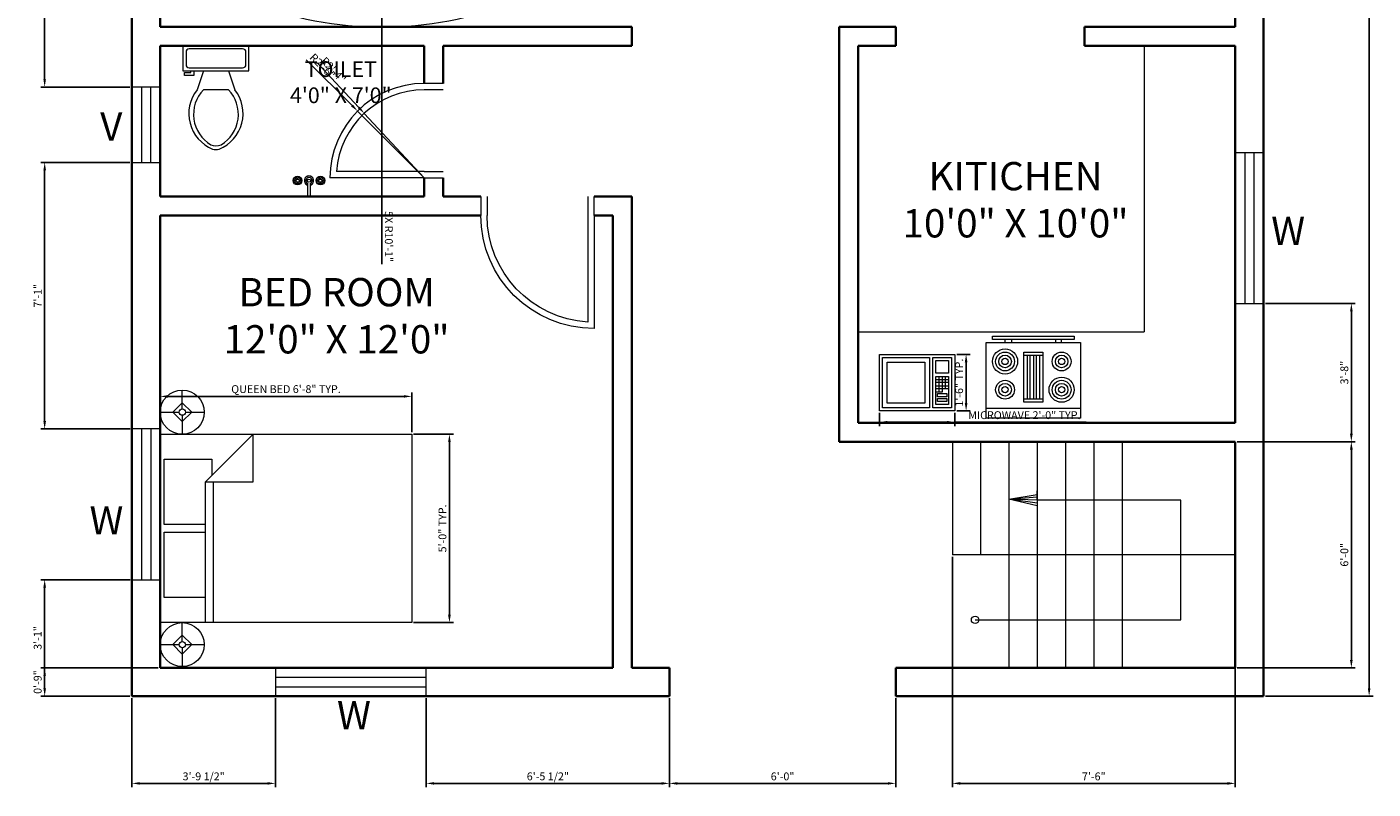
# Model space of a CAD drawing. Units: inches. Extents: x 1025 to 3479, y 1594 to 2212.
# Tile 1 of 9: x 1766 to 2194, y 1601 to 1843. Entities that reach past the tile are written whole.
import ezdxf

# ---------------------------------------------------------------- set-up
doc = ezdxf.new("R2010")
doc.units = ezdxf.units.IN
for name, color, linetype, lineweight in [('A-ANNO-DIMS', 1, 'Continuous', 18), ('A-ANNO-SYMB', 1, 'Continuous', 13), ('A-ANNO-TEXT', 7, 'Continuous', 18), ('A-AREA-IDEN', 4, 'Continuous', 18), ('A-DOOR', 4, 'Continuous', 18), ('A-EQPM', 9, 'Continuous', 18), ('A-FLOR-CSWK', 8, 'Continuous', 18), ('A-FLOR-FIXT', 9, 'Continuous', 18), ('A-FLOR-STRS', 7, 'Continuous', 18), ('A-FURN', 8, 'Continuous', 13), ('A-GLAZ', 3, 'Continuous', 18), ('A-WALL', 7, 'Continuous', 35)]:
    doc.layers.add(name, color=color, linetype=linetype, lineweight=lineweight)
doc.styles.get("Standard").update_dxf_attribs({"font": 'arial.ttf'})
doc.dimstyles.new('ISO-25', dxfattribs={"dimtxt": 2.5, "dimasz": 2.5, "dimexe": 1.25, "dimexo": 0.625, "dimtad": 1, "dimdec": 0, "dimlunit": 3, "dimtxsty": 'Standard', "dimcen": 2.5, "dimadec": 0, "dimazin": 0, "dimtfac": 1, "dimtdec": 0, "dimtmove": 0, "dimatfit": 3, "dimfxl": 1, "dimarcsym": 0})

# ---------------------------------------------------------------- blocks, each defined once
blk = doc.blocks.new('*D4')
at = {"layer": 'A-ANNO-DIMS', "color": 0, "lineweight": -2, "transparency": 16777216}
for p, q in [((2159.72, 2110.49), (2193.95, 2110.49)), ((2192.7, 2107.99), (2192.7, 1632.99)), ((2159.72, 1630.49), (2193.95, 1630.49))]:
    blk.add_line(p, q, dxfattribs=at)
at = {"layer": 'A-ANNO-DIMS', "color": 0, "transparency": 16777216}
for points in [[(2192.28, 2107.99), (2193.12, 2107.99), (2192.7, 2110.49)], [(2192.28, 1632.99), (2193.12, 1632.99), (2192.7, 1630.49)]]:
    blk.add_solid(points, dxfattribs=at)
at = {"layer": 'Defpoints', "color": 0, "transparency": 16777216}
for p in [(2159.1, 2110.49), (2159.1, 1630.49), (2192.7, 1630.49)]:
    blk.add_point(p, dxfattribs=at)
at = {"layer": 'A-ANNO-DIMS', "color": 0, "transparency": 16777216, "insert": (2190.8, 1870.49), "char_height": 2.5, "attachment_point": 5, "rotation": 90}
blk.add_mtext("40'", dxfattribs=at)
blk = doc.blocks.new('Range-Oven - 30 in top')
for p, q in [((0, -3), (30, -3)), ((12, -6), (18, -6)), ((13, -20), (13, -6)), ((14, -6), (14, -20)), ((15, -20), (15, -6)), ((16, -6), (16, -20)), ((17, -20), (17, -6)), ((18, -20), (12, -20)), ((6, -24), (6, -25)), ((8, -25), (8, -24)), ((22, -25), (22, -24)), ((24, -24), (24, -25))]:
    blk.add_line(p, q)
for points in [[(0, -24), (0, 0), (30, 0), (30, -24)], [(12, -21), (12, -5), (18, -5), (18, -21)], [(2, -26), (2, -25), (28, -25), (28, -26)]]:
    blk.add_lwpolyline(points, close=True)
for centre, radius in [((6, -9), 4), ((6, -9), 3), ((6, -9), 2), ((6, -9), 1), ((24, -9), 3), ((24, -9), 2), ((24, -9), 1), ((6, -18), 3), ((6, -18), 2), ((6, -18), 1), ((24, -18), 4), ((24, -18), 3), ((24, -18), 2), ((24, -18), 1)]:
    blk.add_circle(centre, radius)
blk = doc.blocks.new('Sofa - Roundback 7 ft.')
for p, q in [((-12.00002, -32.4421), (-12.00003, -6.5971)), ((11.99997, -32.4421), (11.99998, -6.5971)), ((-36.000027, -34), (-36.000027, -11.4696)), ((35.99998, -34), (35.99998, -11.4696)), ((-35.999844, -13.3819), (35.9998, -13.3819)), ((-36.000027, -32.4421), (35.99998, -32.4421))]:
    blk.add_line(p, q)
for points in [[(-36.000027, -34), (-42.000027, -34), (-42.000027, -8)], [(41.99998, -8), (41.99998, -34), (35.99998, -34)]]:
    blk.add_lwpolyline(points)
for centre, radius, start, end in [((0, -114.25), 114.25, 68.43141, 111.5686), ((-0.00001, -127.1968), 121.1968, 72.72033, 107.2797)]:
    blk.add_arc(centre, radius, start, end)
blk = doc.blocks.new('Bed - Queen')
for p, q in [((0, -80.00003), (0, 0)), ((0, 0), (59.99999, 0)), ((59.99999, 0), (59.99999, -80.00003)), ((7.99999, -1.2), (28.79998, -1.2)), ((7.99999, -14.4), (7.99999, -1.2)), ((28.79998, -1.2), (28.79998, -14.4)), ((31.19999, -1.2), (51.99999, -1.2)), ((31.19999, -14.4), (31.19999, -1.2)), ((51.99999, -1.2), (51.99999, -16.4)), ((0, -14.4), (44.8, -14.4)), ((44.8, -16.8), (0, -16.8)), ((59.99999, -29.6), (44.8, -14.4)), ((44.8, -14.4), (44.8, -29.6)), ((51.99999, -16.4), (46.79936, -16.4)), ((44.8, -29.6), (59.99999, -29.6)), ((59.99999, -80.00003), (0, -80.00003))]:
    blk.add_line(p, q)
blk = doc.blocks.new('Lamp - Table')
for p, q in [((0, 7), (0, 1)), ((-1, 0), (-7, 0)), ((0, 3), (-3, 0)), ((-3, 0), (0, -3)), ((3, 0), (0, 3)), ((0, -3), (3, 0)), ((1, 0), (7, 0)), ((0, -1), (0, -7))]:
    blk.add_line(p, q)
for radius in [7, 1]:
    blk.add_circle((0, 0), radius)
blk = doc.blocks.new('Toilet - top')
for p, q in [((9.5, -6), (9.5, -2)), ((-10, -8.5), (-8, -8.5)), ((-10, -9.5), (-10, -8.5)), ((-8, -8.5), (-8, -8)), ((-7, -8), (-7, -9.5)), ((-4, -8), (-6, -14)), ((4, -8), (6, -14)), ((-7, -9.5), (-10, -9.5)), ((4, -14), (-4, -14))]:
    blk.add_line(p, q)
blk.add_lwpolyline([(10.5, -8), (10.5, 0), (-10.5, 0), (-10.5, -8)], close=True)
for points in [[(-9.5, -2), (-9.5, -6)], [(8.5, -1), (-8.5, -1)], [(-8.5, -7), (8.5, -7)]]:
    blk.add_lwpolyline(points)
for centre, radius, start, end in [((-8.62, -1.88), 0.884, 81.8699, 188.1301), ((8.62, -1.88), 0.884, 351.8699, 98.1301), ((-8.62, -6.12), 0.884, 171.8699, 278.1301), ((8.62, -6.12), 0.884, 261.8699, 8.1301), ((3.52, -21.58), 12.17, 141.4691, 247.9714), ((4.2, -21.82), 11.33, 136.3677, 238.9468), ((-3.52, -21.58), 12.17, 292.0284, 38.5307), ((-4.2, -21.82), 11.33, 301.053, 43.6321), ((0, -27.88), 4, 245.7318, 294.2682), ((0, -29), 4, 254.8605, 285.1395)]:
    blk.add_arc(centre, radius, start, end)
blk = doc.blocks.new('Faucet - Bathroom top')
for p, q in [((-4.107, 0.125), (-4.375, 0.125)), ((-3.75, 0.4788), (-3.75, 0.75)), ((-3.5, 0.482), (-3.5, 0.75)), ((-3.1461, 0.125), (-2.875, 0.125)), ((3.143, 0.125), (2.875, 0.125)), ((3.5, 0.4788), (3.5, 0.75)), ((3.75, 0.482), (3.75, 0.75)), ((4.1039, 0.125), (4.375, 0.125)), ((-4.1039, -0.125), (-4.375, -0.125)), ((-3.75, -0.4821), (-3.75, -0.75)), ((-3.5, -0.4789), (-3.5, -0.75)), ((-3.143, -0.125), (-2.875, -0.125)), ((-0.5, -0.8639), (-0.5, -4.5)), ((0.5, -4.5), (0.5, -0.8631)), ((3.1461, -0.125), (2.875, -0.125)), ((3.5, -0.4821), (3.5, -0.75)), ((3.75, -0.4789), (3.75, -0.75)), ((4.107, -0.125), (4.375, -0.125))]:
    blk.add_line(p, q)
for centre, radius in [((-3.625, 0), 1.375), ((-4.625, 0), 0.2795), ((-3.625, 0), 0.5), ((-3.625, 1), 0.2795), ((-2.625, 0), 0.2795), ((0, 0), 0.5), ((3.625, 0), 1.375), ((2.625, 0), 0.2795), ((3.625, 0), 0.5), ((3.625, 1), 0.2795), ((4.625, 0), 0.2795), ((-3.625, -1), 0.2795), ((3.625, -1), 0.2795)]:
    blk.add_circle(centre, radius)
for centre, radius, start, end in [((-3.625, 0), 1, 105.2407, 164.2093), ((-3.625, 0), 1, 16.44125, 74.07887), ((0, 0), 1.5, 289.6514, 250.3603), ((0, 0), 1, 300.3431, 239.7554), ((3.625, 0), 1, 106.12, 164.0884), ((3.625, 0), 1, 16.23422, 73.90469), ((-3.625, 0), 1, 196.2342, 253.9047), ((-3.625, 0), 1, 286.12, 344.0884), ((3.625, 0), 1, 196.4413, 254.0789), ((3.625, 0), 1, 285.2407, 344.2093), ((0, -4.5), 0.5, 180, 0)]:
    blk.add_arc(centre, radius, start, end)
blk = doc.blocks.new('Microwave')
for p, q in [((18, 10), (22, 10)), ((22, 9), (18, 9)), ((19, 7), (19, 11)), ((20, 11), (20, 7)), ((21, 7), (21, 11)), ((18, 8), (22, 8)), ((22, 7), (18, 7)), ((20, 6), (18, 6)), ((19, 6), (19, 7)), ((20, 7), (20, 6))]:
    blk.add_line(p, q)
for points in [[(0, 0), (0, 18), (24, 18), (24, 0)], [(1, 1), (1, 17), (16, 17), (16, 1)], [(2.5, 2.5), (2.5, 15.5), (14.5, 15.5), (14.5, 2.5)], [(17, 1), (17, 17), (23, 17), (23, 1)], [(18, 12), (18, 16), (22, 16), (22, 12)], [(18, 2), (18, 11), (22, 11), (22, 2)], [(18.5, 4.5), (18.5, 5.5), (21.5, 5.5), (21.5, 4.5)], [(18.5, 3), (18.5, 4), (21.5, 4), (21.5, 3)]]:
    blk.add_lwpolyline(points, close=True)
blk = doc.blocks.new('WIN-48IN')
for p, q in [((0, 48), (0, 0)), ((9, 48), (0, 48)), ((3, 48), (3, 0)), ((6, 0), (6, 48)), ((9, 0), (9, 48)), ((0, 0), (9, 0))]:
    blk.add_line(p, q)
blk = doc.blocks.new('VENT-24IN')
for p, q in [((24, 9), (0, 9)), ((0, 9), (0, 0)), ((24, 0), (24, 9)), ((24, 6), (0, 6)), ((0, 3), (24, 3)), ((0, 0), (24, 0))]:
    blk.add_line(p, q)
blk = doc.blocks.new('DOOR-SWING-36IN')
for p, q in [((0, 36), (6, 36)), ((0, 34), (6, 34)), ((0, 2), (6, 2)), ((6, 0), (0, 0)), ((6, 2), (39.94, 2)), ((6, 0), (42, 0))]:
    blk.add_line(p, q)
for radius, start in [(36, 0), (34, 3.3723)]:
    blk.add_arc((6, 0), radius, start, 90)
blk = doc.blocks.new('*D24')
at = {"layer": 'A-ANNO-DIMS', "color": 0, "lineweight": -2, "transparency": 16777216}
for p, q in [((1808.1, 1714.52), (1808.1, 1727.14)), ((1888.1, 1714.52), (1888.1, 1727.14)), ((1885.6, 1725.89), (1810.6, 1725.89))]:
    blk.add_line(p, q, dxfattribs=at)
at = {"layer": 'A-ANNO-DIMS', "color": 0, "transparency": 16777216}
for points in [[(1810.6, 1726.31), (1810.6, 1725.48), (1808.1, 1725.89)], [(1885.6, 1726.31), (1885.6, 1725.48), (1888.1, 1725.89)]]:
    blk.add_solid(points, dxfattribs=at)
at = {"layer": 'Defpoints', "color": 0, "transparency": 16777216}
for p in [(1808.1, 1725.89), (1808.1, 1713.89), (1888.1, 1713.89)]:
    blk.add_point(p, dxfattribs=at)
at = {"layer": 'A-ANNO-DIMS', "color": 0, "transparency": 16777216, "insert": (1848.1, 1727.89), "char_height": 2.5, "attachment_point": 5}
blk.add_mtext('QUEEN BED 6\'-8" TYP.', dxfattribs=at)
blk = doc.blocks.new('*D25')
at = {"layer": 'A-ANNO-DIMS', "color": 0, "lineweight": -2, "transparency": 16777216}
for p, q in [((1888.72, 1713.89), (1901.35, 1713.89)), ((1900.1, 1656.39), (1900.1, 1711.39)), ((1888.72, 1653.89), (1901.35, 1653.89))]:
    blk.add_line(p, q, dxfattribs=at)
at = {"layer": 'A-ANNO-DIMS', "color": 0, "transparency": 16777216}
for points in [[(1899.68, 1711.39), (1900.52, 1711.39), (1900.1, 1713.89)], [(1899.68, 1656.39), (1900.52, 1656.39), (1900.1, 1653.89)]]:
    blk.add_solid(points, dxfattribs=at)
at = {"layer": 'Defpoints', "color": 0, "transparency": 16777216}
for p in [(1888.1, 1713.89), (1900.1, 1713.89), (1888.1, 1653.89)]:
    blk.add_point(p, dxfattribs=at)
at = {"layer": 'A-ANNO-DIMS', "color": 0, "transparency": 16777216, "insert": (1898.2, 1683.89), "char_height": 2.5, "attachment_point": 5, "rotation": 90}
blk.add_mtext('5\'-0" TYP.', dxfattribs=at)
blk = doc.blocks.new('*D42')
at = {"layer": 'A-ANNO-DIMS', "color": 0, "lineweight": -2, "transparency": 16777216}
for p, q in [((2036.88, 1720.66), (2036.88, 1716.43)), ((2039.38, 1717.68), (2058.38, 1717.68)), ((2060.88, 1720.66), (2060.88, 1716.43)), ((2060.88, 1717.68), (2102.65, 1717.68))]:
    blk.add_line(p, q, dxfattribs=at)
at = {"layer": 'A-ANNO-DIMS', "color": 0, "transparency": 16777216}
for points in [[(2039.38, 1718.1), (2039.38, 1717.27), (2036.88, 1717.68)], [(2058.38, 1718.1), (2058.38, 1717.27), (2060.88, 1717.68)]]:
    blk.add_solid(points, dxfattribs=at)
at = {"layer": 'Defpoints', "color": 0, "transparency": 16777216}
for p in [(2036.88, 1721.28), (2060.88, 1721.28), (2060.88, 1717.68)]:
    blk.add_point(p, dxfattribs=at)
at = {"layer": 'A-ANNO-DIMS', "color": 0, "transparency": 16777216, "insert": (2083.02, 1719.6), "char_height": 2.5, "attachment_point": 5}
blk.add_mtext('MICROWAVE 2\'-0" TYP.', dxfattribs=at)
blk = doc.blocks.new('*D43')
at = {"layer": 'A-ANNO-DIMS', "color": 0, "lineweight": -2, "transparency": 16777216}
for p, q in [((2061.51, 1739.28), (2065.73, 1739.28)), ((2064.48, 1723.78), (2064.48, 1736.78)), ((2061.51, 1721.28), (2065.73, 1721.28))]:
    blk.add_line(p, q, dxfattribs=at)
at = {"layer": 'A-ANNO-DIMS', "color": 0, "transparency": 16777216}
for points in [[(2064.06, 1736.78), (2064.9, 1736.78), (2064.48, 1739.28)], [(2064.06, 1723.78), (2064.9, 1723.78), (2064.48, 1721.28)]]:
    blk.add_solid(points, dxfattribs=at)
at = {"layer": 'Defpoints', "color": 0, "transparency": 16777216}
for p in [(2060.88, 1739.28), (2064.48, 1739.28), (2060.88, 1721.28)]:
    blk.add_point(p, dxfattribs=at)
at = {"layer": 'A-ANNO-DIMS', "color": 0, "transparency": 16777216, "insert": (2062.58, 1730.28), "char_height": 2.5, "attachment_point": 5, "rotation": 90}
blk.add_mtext('1\'-6" TYP.', dxfattribs=at)
blk = doc.blocks.new('*D46')
at = {"layer": 'A-ANNO-DIMS', "color": 0, "lineweight": -2, "transparency": 16777216}
for p, q in [((1970.1, 1629.86), (1970.1, 1601.49)), ((2042.1, 1629.86), (2042.1, 1601.49)), ((1972.6, 1602.74), (2039.6, 1602.74))]:
    blk.add_line(p, q, dxfattribs=at)
at = {"layer": 'A-ANNO-DIMS', "color": 0, "transparency": 16777216}
for points in [[(1972.6, 1603.15), (1972.6, 1602.32), (1970.1, 1602.74)], [(2039.6, 1603.15), (2039.6, 1602.32), (2042.1, 1602.74)]]:
    blk.add_solid(points, dxfattribs=at)
at = {"layer": 'Defpoints', "color": 0, "transparency": 16777216}
for p in [(1970.1, 1630.49), (2042.1, 1630.49), (2042.1, 1602.74)]:
    blk.add_point(p, dxfattribs=at)
at = {"layer": 'A-ANNO-DIMS', "color": 0, "transparency": 16777216, "insert": (2006.1, 1604.64), "char_height": 2.5, "attachment_point": 5}
blk.add_mtext('6\'-0"', dxfattribs=at)
blk = doc.blocks.new('*D52')
at = {"layer": 'A-ANNO-DIMS', "color": 0, "lineweight": -2, "transparency": 16777216}
for p, q in [((1798.57, 1667.55), (1770.08, 1667.55)), ((1771.33, 1632.99), (1771.33, 1665.05)), ((1798.47, 1630.49), (1770.08, 1630.49))]:
    blk.add_line(p, q, dxfattribs=at)
at = {"layer": 'A-ANNO-DIMS', "color": 0, "transparency": 16777216}
for points in [[(1770.92, 1665.05), (1771.75, 1665.05), (1771.33, 1667.55)], [(1770.92, 1632.99), (1771.75, 1632.99), (1771.33, 1630.49)]]:
    blk.add_solid(points, dxfattribs=at)
at = {"layer": 'Defpoints', "color": 0, "transparency": 16777216}
for p in [(1771.33, 1667.55), (1799.19, 1667.55), (1799.1, 1630.49)]:
    blk.add_point(p, dxfattribs=at)
at = {"layer": 'A-ANNO-DIMS', "color": 0, "transparency": 16777216, "insert": (1769.43, 1649.02), "char_height": 2.5, "attachment_point": 5, "rotation": 90}
blk.add_mtext('3\'-1"', dxfattribs=at)
blk = doc.blocks.new('*D53')
at = {"layer": 'A-ANNO-DIMS', "color": 0, "lineweight": -2, "transparency": 16777216}
for p, q in [((1798.47, 1800.34), (1770.08, 1800.34)), ((1771.33, 1718.05), (1771.33, 1797.84)), ((1798.57, 1715.55), (1770.08, 1715.55))]:
    blk.add_line(p, q, dxfattribs=at)
at = {"layer": 'A-ANNO-DIMS', "color": 0, "transparency": 16777216}
for points in [[(1770.92, 1797.84), (1771.75, 1797.84), (1771.33, 1800.34)], [(1770.92, 1718.05), (1771.75, 1718.05), (1771.33, 1715.55)]]:
    blk.add_solid(points, dxfattribs=at)
at = {"layer": 'Defpoints', "color": 0, "transparency": 16777216}
for p in [(1771.33, 1800.34), (1799.1, 1800.34), (1799.19, 1715.55)]:
    blk.add_point(p, dxfattribs=at)
at = {"layer": 'A-ANNO-DIMS', "color": 0, "transparency": 16777216, "insert": (1769.45, 1757.94), "char_height": 2.5, "attachment_point": 5, "rotation": 90}
blk.add_mtext('7\'-1"', dxfattribs=at)
blk = doc.blocks.new('*D54')
at = {"layer": 'A-ANNO-DIMS', "color": 0, "lineweight": -2, "transparency": 16777216}
for p, q in [((1798.47, 1887.99), (1770.08, 1887.99)), ((1771.33, 1826.84), (1771.33, 1885.49)), ((1798.47, 1824.34), (1770.08, 1824.34))]:
    blk.add_line(p, q, dxfattribs=at)
at = {"layer": 'A-ANNO-DIMS', "color": 0, "transparency": 16777216}
for points in [[(1770.92, 1885.49), (1771.75, 1885.49), (1771.33, 1887.99)], [(1770.92, 1826.84), (1771.75, 1826.84), (1771.33, 1824.34)]]:
    blk.add_solid(points, dxfattribs=at)
at = {"layer": 'Defpoints', "color": 0, "transparency": 16777216}
for p in [(1771.33, 1887.99), (1799.1, 1887.99), (1799.1, 1824.34)]:
    blk.add_point(p, dxfattribs=at)
at = {"layer": 'A-ANNO-DIMS', "color": 0, "transparency": 16777216, "insert": (1769.41, 1856.16), "char_height": 2.5, "attachment_point": 5, "rotation": 90}
blk.add_mtext('5\'-3 1/2"', dxfattribs=at)
blk = doc.blocks.new('*D67')
at = {"layer": 'A-ANNO-DIMS', "color": 0, "lineweight": -2, "transparency": 16777216}
for p, q in [((1807.47, 1639.49), (1770.08, 1639.49)), ((1771.33, 1632.99), (1771.33, 1636.99)), ((1798.47, 1630.49), (1770.08, 1630.49))]:
    blk.add_line(p, q, dxfattribs=at)
at = {"layer": 'A-ANNO-DIMS', "color": 0, "transparency": 16777216}
for points in [[(1770.92, 1636.99), (1771.75, 1636.99), (1771.33, 1639.49)], [(1770.92, 1632.99), (1771.75, 1632.99), (1771.33, 1630.49)]]:
    blk.add_solid(points, dxfattribs=at)
at = {"layer": 'Defpoints', "color": 0, "transparency": 16777216}
for p in [(1771.33, 1639.49), (1808.1, 1639.49), (1799.1, 1630.49)]:
    blk.add_point(p, dxfattribs=at)
at = {"layer": 'A-ANNO-DIMS', "color": 0, "transparency": 16777216, "insert": (1769.43, 1634.99), "char_height": 2.5, "attachment_point": 5, "rotation": 90}
blk.add_mtext('0\'-9"', dxfattribs=at)
blk = doc.blocks.new('*D71')
at = {"layer": 'A-ANNO-DIMS', "color": 0, "lineweight": -2, "transparency": 16777216}
for p, q in [((2159.72, 1755.46), (2188.29, 1755.46)), ((2187.04, 1713.99), (2187.04, 1752.96)), ((2150.72, 1711.49), (2188.29, 1711.49))]:
    blk.add_line(p, q, dxfattribs=at)
at = {"layer": 'A-ANNO-DIMS', "color": 0, "transparency": 16777216}
for points in [[(2186.62, 1752.96), (2187.46, 1752.96), (2187.04, 1755.46)], [(2186.62, 1713.99), (2187.46, 1713.99), (2187.04, 1711.49)]]:
    blk.add_solid(points, dxfattribs=at)
at = {"layer": 'Defpoints', "color": 0, "transparency": 16777216}
for p in [(2159.1, 1755.46), (2187.04, 1755.46), (2150.1, 1711.49)]:
    blk.add_point(p, dxfattribs=at)
at = {"layer": 'A-ANNO-DIMS', "color": 0, "transparency": 16777216, "insert": (2185.14, 1733.47), "char_height": 2.5, "attachment_point": 5, "rotation": 90}
blk.add_mtext('3\'-8"', dxfattribs=at)
blk = doc.blocks.new('*D72')
at = {"layer": 'A-ANNO-DIMS', "color": 0, "lineweight": -2, "transparency": 16777216}
for p, q in [((1799.1, 1629.86), (1799.1, 1601.49)), ((1844.74, 1629.86), (1844.74, 1601.49)), ((1801.6, 1602.74), (1842.24, 1602.74))]:
    blk.add_line(p, q, dxfattribs=at)
at = {"layer": 'A-ANNO-DIMS', "color": 0, "transparency": 16777216}
for points in [[(1801.6, 1603.15), (1801.6, 1602.32), (1799.1, 1602.74)], [(1842.24, 1603.15), (1842.24, 1602.32), (1844.74, 1602.74)]]:
    blk.add_solid(points, dxfattribs=at)
at = {"layer": 'Defpoints', "color": 0, "transparency": 16777216}
for p in [(1799.1, 1630.49), (1844.74, 1630.49), (1844.74, 1602.74)]:
    blk.add_point(p, dxfattribs=at)
at = {"layer": 'A-ANNO-DIMS', "color": 0, "transparency": 16777216, "insert": (1821.92, 1604.65), "char_height": 2.5, "attachment_point": 5}
blk.add_mtext('3\'-9 1/2"', dxfattribs=at)
blk = doc.blocks.new('*D73')
at = {"layer": 'A-ANNO-DIMS', "color": 0, "lineweight": -2, "transparency": 16777216}
for p, q in [((1892.74, 1629.86), (1892.74, 1601.49)), ((1970.1, 1629.86), (1970.1, 1601.49)), ((1895.24, 1602.74), (1967.6, 1602.74))]:
    blk.add_line(p, q, dxfattribs=at)
at = {"layer": 'A-ANNO-DIMS', "color": 0, "transparency": 16777216}
for points in [[(1895.24, 1603.15), (1895.24, 1602.32), (1892.74, 1602.74)], [(1967.6, 1603.15), (1967.6, 1602.32), (1970.1, 1602.74)]]:
    blk.add_solid(points, dxfattribs=at)
at = {"layer": 'Defpoints', "color": 0, "transparency": 16777216}
for p in [(1892.74, 1630.49), (1970.1, 1630.49), (1970.1, 1602.74)]:
    blk.add_point(p, dxfattribs=at)
at = {"layer": 'A-ANNO-DIMS', "color": 0, "transparency": 16777216, "insert": (1931.42, 1604.65), "char_height": 2.5, "attachment_point": 5}
blk.add_mtext('6\'-5 1/2"', dxfattribs=at)
blk = doc.blocks.new('*D78')
at = {"layer": 'A-ANNO-DIMS', "color": 0, "lineweight": -2, "transparency": 16777216}
for p, q in [((2060.1, 1674.86), (2060.1, 1601.49)), ((2150.1, 1674.86), (2150.1, 1601.49)), ((2062.6, 1602.74), (2147.6, 1602.74))]:
    blk.add_line(p, q, dxfattribs=at)
at = {"layer": 'A-ANNO-DIMS', "color": 0, "transparency": 16777216}
for points in [[(2062.6, 1603.15), (2062.6, 1602.32), (2060.1, 1602.74)], [(2147.6, 1603.15), (2147.6, 1602.32), (2150.1, 1602.74)]]:
    blk.add_solid(points, dxfattribs=at)
at = {"layer": 'Defpoints', "color": 0, "transparency": 16777216}
for p in [(2060.1, 1675.49), (2150.1, 1675.49), (2150.1, 1602.74)]:
    blk.add_point(p, dxfattribs=at)
at = {"layer": 'A-ANNO-DIMS', "color": 0, "transparency": 16777216, "insert": (2105.1, 1604.64), "char_height": 2.5, "attachment_point": 5}
blk.add_mtext('7\'-6"', dxfattribs=at)
blk = doc.blocks.new('*D79')
at = {"layer": 'A-ANNO-DIMS', "color": 0, "lineweight": -2, "transparency": 16777216}
for p, q in [((2150.72, 1711.49), (2188.29, 1711.49)), ((2187.04, 1641.99), (2187.04, 1708.99)), ((2150.72, 1639.49), (2188.29, 1639.49))]:
    blk.add_line(p, q, dxfattribs=at)
at = {"layer": 'A-ANNO-DIMS', "color": 0, "transparency": 16777216}
for points in [[(2186.62, 1708.99), (2187.46, 1708.99), (2187.04, 1711.49)], [(2186.62, 1641.99), (2187.46, 1641.99), (2187.04, 1639.49)]]:
    blk.add_solid(points, dxfattribs=at)
at = {"layer": 'Defpoints', "color": 0, "transparency": 16777216}
for p in [(2150.1, 1711.49), (2187.04, 1711.49), (2150.1, 1639.49)]:
    blk.add_point(p, dxfattribs=at)
at = {"layer": 'A-ANNO-DIMS', "color": 0, "transparency": 16777216, "insert": (2185.14, 1675.49), "char_height": 2.5, "attachment_point": 5, "rotation": 90}
blk.add_mtext('6\'-0"', dxfattribs=at)
blk = doc.blocks.new('*D89')
at = {"layer": 'A-ANNO-DIMS', "color": 0, "lineweight": -2, "transparency": 16777216}
for p, q in [((1854.52, 1833.06), (1869.12, 1818.47)), ((1892.1, 1795.49), (1870.89, 1816.7))]:
    blk.add_line(p, q, dxfattribs=at)
at = {"layer": 'A-ANNO-DIMS', "color": 0, "transparency": 16777216}
blk.add_solid([(1869.41, 1818.76), (1868.82, 1818.17), (1870.89, 1816.7)], dxfattribs=at)
at = {"layer": 'Defpoints', "color": 0, "transparency": 16777216}
for p in [(1870.89, 1816.7), (1892.1, 1795.49)]:
    blk.add_point(p, dxfattribs=at)
at = {"layer": 'A-ANNO-DIMS', "color": 0, "transparency": 16777216, "insert": (1859.5, 1830.77), "char_height": 2.5, "attachment_point": 5, "rotation": 314.9994}
blk.add_mtext('R2\'-6"', dxfattribs=at)
blk = doc.blocks.new('*D90')
at = {"layer": 'A-ANNO-DIMS', "color": 0, "lineweight": -2, "transparency": 16777216}
for p, q in [((1878.6, 1970.65), (1878.6, 1849.46)), ((1878.6, 1767.94), (1878.6, 1846.96))]:
    blk.add_line(p, q, dxfattribs=at)
at = {"layer": 'A-ANNO-DIMS', "color": 0, "transparency": 16777216}
blk.add_solid([(1879.02, 1846.96), (1878.18, 1846.96), (1878.6, 1849.46)], dxfattribs=at)
at = {"layer": 'Defpoints', "color": 0, "transparency": 16777216}
for p in [(1878.6, 1970.65), (1878.6, 1849.46)]:
    blk.add_point(p, dxfattribs=at)
at = {"layer": 'A-ANNO-DIMS', "color": 0, "transparency": 16777216, "insert": (1880.5, 1776.74), "char_height": 2.5, "attachment_point": 5, "rotation": 270.0002}
blk.add_mtext('5X R10\'-1"', dxfattribs=at)
blk = doc.blocks.new('*D98')
at = {"layer": 'A-ANNO-DIMS', "color": 0, "lineweight": -2, "transparency": 16777216}
for p, q in [((1858.07, 1832.04), (1871.32, 1817.81)), ((1892.1, 1795.49), (1873.02, 1815.98))]:
    blk.add_line(p, q, dxfattribs=at)
at = {"layer": 'A-ANNO-DIMS', "color": 0, "transparency": 16777216}
blk.add_solid([(1871.62, 1818.09), (1871.01, 1817.52), (1873.02, 1815.98)], dxfattribs=at)
at = {"layer": 'Defpoints', "color": 0, "transparency": 16777216}
for p in [(1873.02, 1815.98), (1892.1, 1795.49)]:
    blk.add_point(p, dxfattribs=at)
at = {"layer": 'A-ANNO-DIMS', "color": 0, "transparency": 16777216, "insert": (1862.95, 1829.56), "char_height": 2.5, "attachment_point": 5, "rotation": 312.953}
blk.add_mtext('R2\'-4"', dxfattribs=at)

msp = doc.modelspace()

# ---------------------------------------------------------------- linework, layer by layer
at = {"layer": 'A-ANNO-SYMB'}
for p, q in [((2078.1, 1693.15), (2087.1, 1694.7)), ((2078.1, 1693.15), (2087.1, 1693.96)), ((2087.1, 1691.12), (2078.1, 1693.15)), ((2087.1, 1692.86), (2078.1, 1693.15)), ((2087.1, 1691.94), (2078.1, 1693.15)), ((2087.1, 1692.86), (2087.1, 1695.86)), ((2087.1, 1695.86), (2087.1, 1692.86)), ((2087.1, 1694.36), (2087.1, 1694.7)), ((2087.1, 1693.96), (2087.1, 1691.94)), ((2132.8, 1692.86), (2087.1, 1692.86)), ((2087.1, 1692.86), (2087.1, 1689.86)), ((2132.8, 1654.79), (2132.8, 1692.86)), ((2067.35, 1654.79), (2132.8, 1654.79))]:
    msp.add_line(p, q, dxfattribs=at)
msp.add_circle((2067.35, 1654.79), 1.2, dxfattribs=at)
at = {"layer": 'A-DOOR'}
for p, q in [((1898.1, 1825.49), (1892.1, 1825.49)), ((1898.1, 1823.49), (1892.1, 1823.49)), ((1892.1, 1795.49), (1862.1, 1795.49)), ((1892.1, 1797.49), (1864.17, 1797.49)), ((1892.1, 1797.49), (1898.1, 1797.49)), ((1892.1, 1795.49), (1898.1, 1795.49))]:
    msp.add_line(p, q, dxfattribs=at)
for radius, end in [(30, 180), (28, 175.904)]:
    msp.add_arc((1892.1, 1795.49), radius, 90, end, dxfattribs=at)
at = {"layer": 'A-FLOR-CSWK'}
for p, q in [((2121.1, 1837.49), (2121.1, 1763.49)), ((2121.1, 1763.49), (2121.1, 1759.49)), ((2121.1, 1759.49), (2121.1, 1746.49)), ((2030.1, 1746.49), (2121.1, 1746.49))]:
    msp.add_line(p, q, dxfattribs=at)
at = {"layer": 'A-FLOR-STRS'}
for p, q in [((2060.1, 1711.49), (2060.1, 1675.49)), ((2069.1, 1711.49), (2069.1, 1675.49)), ((2078.1, 1711.49), (2078.1, 1639.49)), ((2087.1, 1711.49), (2087.1, 1639.49)), ((2096.1, 1711.49), (2096.1, 1639.49)), ((2105.1, 1711.49), (2105.1, 1639.49)), ((2114.1, 1711.49), (2114.1, 1639.49)), ((2150.1, 1675.49), (2060.1, 1675.49))]:
    msp.add_line(p, q, dxfattribs=at)
at = {"layer": 'A-WALL'}
for p, q in [((1799.1, 1670.49), (1799.1, 2110.49)), ((1799.1, 1670.49), (1799.1, 2110.49)), ((2159.1, 2110.49), (2159.1, 1630.49)), ((1808.1, 1843.49), (1808.1, 1963.49)), ((2150.1, 1963.49), (2150.1, 1843.49)), ((1808.1, 1843.49), (1958.1, 1843.49)), ((1958.1, 1837.49), (1958.1, 1843.49)), ((2024.1, 1843.49), (2042.1, 1843.49)), ((2024.1, 1837.49), (2024.1, 1843.49)), ((2042.1, 1837.49), (2042.1, 1843.49)), ((2102.1, 1843.49), (2102.1, 1837.49)), ((2102.1, 1843.49), (2150.1, 1843.49)), ((1808.1, 1837.49), (1892.1, 1837.49)), ((1808.1, 1789.49), (1808.1, 1837.49)), ((1892.1, 1825.49), (1892.1, 1837.49)), ((1898.1, 1837.49), (1952.1, 1837.49)), ((1898.1, 1825.49), (1898.1, 1837.49)), ((1952.1, 1837.49), (1958.1, 1837.49)), ((2024.1, 1837.49), (2024.1, 1763.49)), ((2030.1, 1837.49), (2042.1, 1837.49)), ((2030.1, 1837.49), (2030.1, 1763.49)), ((2030.1, 1837.49), (2042.1, 1837.49)), ((2102.1, 1837.49), (2150.1, 1837.49)), ((2150.1, 1837.49), (2150.1, 1763.49)), ((1892.1, 1789.49), (1892.1, 1795.49)), ((1892.1, 1789.49), (1892.1, 1795.49)), ((1898.1, 1789.49), (1898.1, 1795.49)), ((1808.1, 1789.49), (1892.1, 1789.49)), ((1898.1, 1789.49), (1910.1, 1789.49)), ((1946.1, 1789.49), (1952.1, 1789.49)), ((1952.1, 1789.49), (1958.1, 1789.49)), ((1958.1, 1670.49), (1958.1, 1789.49)), ((1808.1, 1670.49), (1808.1, 1783.49)), ((1808.1, 1783.49), (1910.1, 1783.49)), ((1952.1, 1783.49), (1946.1, 1783.49)), ((1946.1, 1783.49), (1952.1, 1783.49)), ((1952.1, 1670.49), (1952.1, 1783.49)), ((1952.1, 1670.49), (1952.1, 1783.49)), ((2024.1, 1763.49), (2024.1, 1759.49)), ((2030.1, 1763.49), (2030.1, 1759.49)), ((2150.1, 1763.49), (2150.1, 1759.49)), ((2024.1, 1759.49), (2024.1, 1711.49)), ((2030.1, 1759.49), (2030.1, 1717.49)), ((2150.1, 1759.49), (2150.1, 1717.49)), ((2030.1, 1717.49), (2150.1, 1717.49)), ((2030.1, 1711.49), (2024.1, 1711.49)), ((2030.1, 1711.49), (2150.1, 1711.49)), ((2150.1, 1711.49), (2150.1, 1639.49)), ((1799.1, 1630.49), (1799.1, 1670.49)), ((1808.1, 1639.49), (1808.1, 1670.49)), ((1952.1, 1639.49), (1952.1, 1670.49)), ((1958.1, 1639.49), (1958.1, 1670.49)), ((1952.1, 1639.49), (1808.1, 1639.49)), ((1970.1, 1639.49), (1958.1, 1639.49)), ((1958.1, 1639.49), (1970.1, 1639.49)), ((1970.1, 1639.49), (1970.1, 1630.49)), ((2150.1, 1639.49), (2042.1, 1639.49)), ((2042.1, 1630.49), (2042.1, 1639.49)), ((1970.1, 1630.49), (1799.1, 1630.49)), ((2159.1, 1630.49), (2042.1, 1630.49))]:
    msp.add_line(p, q, dxfattribs=at)

# ---------------------------------------------------------------- block references
at = {"layer": 'A-DOOR', "extrusion": (0, 0, -1), "zscale": -1, "rotation": 269.9999999999993}
msp.add_blockref('DOOR-SWING-36IN', (-1946.1, 1789.49), dxfattribs=at)
at = {"layer": 'A-EQPM', "rotation": 180}
msp.add_blockref('Range-Oven - 30 in top', (2100.87, 1719.02), dxfattribs=at)
at = {"layer": 'A-EQPM'}
msp.add_blockref('Microwave', (2036.88, 1721.28), dxfattribs=at)
at = {"layer": 'A-FLOR-FIXT'}
for name, p in [('Toilet - top', (1825.82, 1837.49)), ('Faucet - Bathroom top', (1855.42, 1794.57))]:
    msp.add_blockref(name, p, dxfattribs=at)
at = {"layer": 'A-FURN'}
for name, p, rotation in [('Sofa - Roundback 7 ft.', (1878.6, 1843.46), 180), ('Lamp - Table', (1815.1, 1720.89), 90), ('Bed - Queen', (1808.1, 1653.89), 90), ('Lamp - Table', (1815.1, 1646.89), 90)]:
    msp.add_blockref(name, p, dxfattribs=dict(at, rotation=rotation))
at = {"layer": 'A-GLAZ'}
for name, p, rotation in [('VENT-24IN', (1799.1, 1824.34), 270.0000000000027), ('WIN-48IN', (1844.74, 1639.49), 269.9999999999999)]:
    msp.add_blockref(name, p, dxfattribs=dict(at, rotation=rotation))
for p in [(2150.1, 1755.46), (1799.19, 1667.55)]:
    msp.add_blockref('WIN-48IN', p, dxfattribs=at)

# ---------------------------------------------------------------- texts
at = {"layer": 'A-ANNO-TEXT', "char_height": 9, "attachment_point": 1}
for s, width, insert in [('\\pxqc;{V}', 7.8272, (1788.6, 1816.29)), ('\\pxqc;W', 15.8719, (2158.99, 1783.06)), ('\\pxqc;W', 15.8719, (1783.04, 1690.96)), ('\\pxqc;W', 15.8719, (1861.79, 1628.91))]:
    msp.add_mtext_dynamic_manual_height_columns(s, width=width, gutter_width=12.5, heights=[0], dxfattribs=dict(at, insert=insert))
at = {"layer": 'A-AREA-IDEN', "attachment_point": 1}
for s, width, insert, char_height in [('\\pxqc;TOILET \\P4\'0" X 7\'0" ', 51.1118, (1840, 1832.56), 5), ('\\pxqc;KITICHEN\\P10\'0" X 10\'0"', 112.2145, (2024.1, 1800.49), 9), ('\\pxqc;BED ROOM \\P12\'0" X 12\'0"', 112.2145, (1808.1, 1763.57), 9)]:
    msp.add_mtext_dynamic_manual_height_columns(s, width=width, gutter_width=12.5, heights=[0], dxfattribs=dict(at, insert=insert, char_height=char_height))

# ---------------------------------------------------------------- dimensions: what is measured, and where the dimension line sits
at = {"layer": 'A-ANNO-DIMS'}
for base, p1, p2, override, picture, middle in [((2192.7, 1630.49), (2159.1, 2110.49), (2159.1, 1630.49), {"dimclrd": 0, "dimclre": 0, "dimclrt": 0}, '*D4', (2190.8, 1870.49)), ((1771.332537, 1887.985569), (1799.099068, 1824.335569), (1799.099068, 1887.985569), {"dimdec": 1, "dimlfac": 1, "dimrnd": 0, "dimzin": 1, "dimdsep": 46, "dimlunit": 4, "dimfrac": 2}, '*D54', (1769.41405132, 1856.160569)), ((1771.33, 1800.34), (1799.19, 1715.55), (1799.1, 1800.34), {"dimdec": 1, "dimlfac": 1, "dimrnd": 0, "dimzin": 1, "dimdsep": 46, "dimlunit": 4, "dimfrac": 2}, '*D53', (1769.45, 1757.94)), ((2187.04, 1755.46), (2150.1, 1711.49), (2159.1, 1755.46), {"dimdec": 1, "dimlfac": 1, "dimrnd": 0, "dimzin": 1, "dimdsep": 46, "dimlunit": 4, "dimfrac": 2}, '*D71', (2185.14, 1733.47)), ((2187.04, 1711.49), (2150.1, 1639.49), (2150.1, 1711.49), {"dimdec": 1, "dimlfac": 1, "dimrnd": 0, "dimzin": 1, "dimdsep": 46, "dimlunit": 4, "dimfrac": 2}, '*D79', (2185.14, 1675.49)), ((1771.33, 1667.55), (1799.1, 1630.49), (1799.19, 1667.55), {"dimdec": 1, "dimlfac": 1, "dimrnd": 0, "dimzin": 1, "dimdsep": 46, "dimlunit": 4, "dimfrac": 2}, '*D52', (1769.43, 1649.02)), ((1771.33, 1639.49), (1799.1, 1630.49), (1808.1, 1639.49), {"dimdec": 1, "dimlfac": 1, "dimrnd": 0, "dimzin": 1, "dimdsep": 46, "dimlunit": 4, "dimfrac": 2}, '*D67', (1769.43, 1634.99))]:
    dim = msp.add_linear_dim(base=base, p1=p1, p2=p2, angle=90, dimstyle='ISO-25', override=override, dxfattribs=at)
    dim.commit()
    dim.dimension.update_dxf_attribs({"geometry": picture, "text_midpoint": middle})
dim = msp.add_radius_dim(center=(1878.6, 1970.65), mpoint=(1878.6, 1849.46), text='5X <>', dimstyle='ISO-25', override={"dimdec": 1, "dimlfac": 1, "dimrnd": 0, "dimzin": 1, "dimdsep": 46, "dimlunit": 4, "dimfrac": 2}, dxfattribs=at)
dim.commit()
dim.dimension.update_dxf_attribs({"geometry": '*D90', "text_midpoint": (1878.6, 1776.74), "dimtype": 164})
for mpoint, picture, middle in [((1870.89, 1816.7), '*D89', (1858.16, 1829.43)), ((1873.02, 1815.98), '*D98', (1861.57, 1828.28))]:
    dim = msp.add_radius_dim(center=(1892.1, 1795.49), mpoint=mpoint, dimstyle='ISO-25', override={"dimdec": 1, "dimlfac": 1, "dimrnd": 0, "dimzin": 1, "dimdsep": 46, "dimlunit": 4, "dimfrac": 2}, dxfattribs=at)
    dim.commit()
    dim.dimension.update_dxf_attribs({"geometry": picture, "text_midpoint": middle, "dimtype": 164})
for base, p1, p2, angle, text, picture, middle in [((2064.48, 1739.28), (2060.88, 1721.28), (2060.88, 1739.28), 90, '<> TYP.', '*D43', (2062.58, 1730.28)), ((1808.1, 1725.89), (1888.1, 1713.89), (1808.1, 1713.89), 180, 'QUEEN BED <> TYP.', '*D24', (1848.1, 1727.89)), ((1900.1, 1713.89), (1888.1, 1653.89), (1888.1, 1713.89), 90, '<> TYP.', '*D25', (1898.2, 1683.89))]:
    dim = msp.add_linear_dim(base=base, p1=p1, p2=p2, angle=angle, text=text, dimstyle='ISO-25', override={"dimdec": 1, "dimlfac": 1, "dimrnd": 0, "dimzin": 1, "dimdsep": 46, "dimlunit": 4, "dimfrac": 2}, dxfattribs=at)
    dim.commit()
    dim.dimension.update_dxf_attribs({"geometry": picture, "text_midpoint": middle})
dim = msp.add_linear_dim(base=(2060.88, 1717.68), p1=(2036.88, 1721.28), p2=(2060.88, 1721.28), text='MICROWAVE <> TYP.', dimstyle='ISO-25', override={"dimdec": 1, "dimlfac": 1, "dimrnd": 0, "dimzin": 1, "dimdsep": 46, "dimlunit": 4, "dimfrac": 2}, dxfattribs=at)
dim.commit()
dim.dimension.update_dxf_attribs({"geometry": '*D42', "text_midpoint": (2083.02, 1719.6)})
for base, p1, p2, picture, middle in [((2150.1, 1602.74), (2060.1, 1675.49), (2150.1, 1675.49), '*D78', (2105.1, 1604.64)), ((1844.74, 1602.74), (1799.1, 1630.49), (1844.74, 1630.49), '*D72', (1821.92, 1604.65)), ((1970.1, 1602.74), (1892.74, 1630.49), (1970.1, 1630.49), '*D73', (1931.42, 1604.65)), ((2042.1, 1602.74), (1970.1, 1630.49), (2042.1, 1630.49), '*D46', (2006.1, 1604.64))]:
    dim = msp.add_linear_dim(base=base, p1=p1, p2=p2, dimstyle='ISO-25', override={"dimdec": 1, "dimlfac": 1, "dimrnd": 0, "dimzin": 1, "dimdsep": 46, "dimlunit": 4, "dimfrac": 2}, dxfattribs=at)
    dim.commit()
    dim.dimension.update_dxf_attribs({"geometry": picture, "text_midpoint": middle})

doc.saveas('drawing.dxf')
